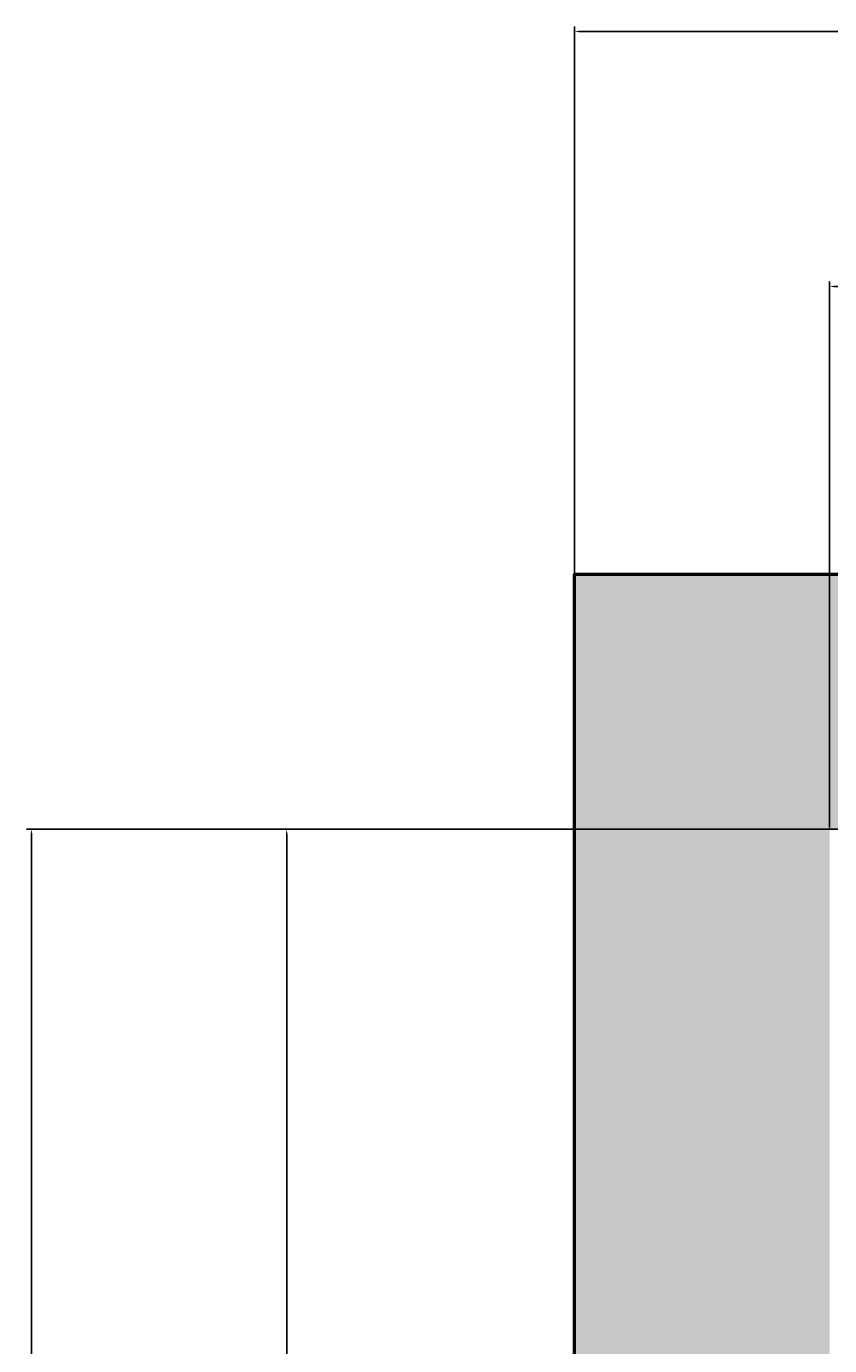
# Model space of a CAD drawing. Units: inches. Extents: x 2307 to 2544, y 2171 to 2540.
# Tile 23 of 52: x 2307 to 2336, y 2493 to 2540. Entities that reach past the tile are written whole.
import ezdxf

# ---------------------------------------------------------------- set-up
doc = ezdxf.new("R2010")
doc.units = ezdxf.units.IN
doc.layers.add('A-ANNO-DIMS', color=2, linetype='Continuous', lineweight=18)
doc.layers.add('A-WALL', color=7, linetype='Continuous', lineweight=50)
doc.layers.add('A-WALL-PATT', color=18, linetype='Continuous', lineweight=13, true_color=0x000000)
doc.styles.get("Standard").update_dxf_attribs({"font": 'arial.ttf'})
doc.dimstyles.get("Standard").update_dxf_attribs({"dimtxt": 0.18, "dimasz": 0.18, "dimexe": 0.18, "dimexo": 0.0625, "dimgap": 0.09, "dimtad": 0, "dimtih": 1, "dimtoh": 1, "dimdec": 4, "dimzin": 0, "dimdsep": 46, "dimtxsty": 'Standard', "dimcen": 0.09, "dimadec": 0, "dimazin": 0, "dimtfac": 1, "dimtdec": 4, "dimtofl": 0, "dimtmove": 0, "dimatfit": 3, "dimfxl": 1, "dimtolj": 1, "dimtzin": 0, "dimarcsym": 0})

# ---------------------------------------------------------------- blocks, each defined once
blk = doc.blocks.new('*D42')
at = {"layer": 'A-ANNO-DIMS', "color": 0, "lineweight": -2, "transparency": 16777216}
for p, q in [((2326.696, 2520.572), (2326.696, 2539.84)), ((2326.876, 2539.66), (2346.669, 2539.66)), ((2367.223, 2539.66), (2347.429, 2539.66)), ((2367.403, 2520.572), (2367.403, 2539.84))]:
    blk.add_line(p, q, dxfattribs=at)
at = {"layer": 'A-ANNO-DIMS', "color": 0, "transparency": 16777216}
for points in [[(2326.876, 2539.69), (2326.876, 2539.63), (2326.696, 2539.66)], [(2367.223, 2539.69), (2367.223, 2539.63), (2367.403, 2539.66)]]:
    blk.add_solid(points, dxfattribs=at)
at = {"layer": 'Defpoints', "color": 0, "transparency": 16777216}
for p in [(2367.403, 2539.66), (2326.696, 2520.51), (2367.403, 2520.51)]:
    blk.add_point(p, dxfattribs=at)
at = {"layer": 'A-ANNO-DIMS', "color": 0, "transparency": 16777216, "insert": (2347.049, 2539.66), "char_height": 0.18, "attachment_point": 5}
blk.add_mtext('\\A1;40.71', dxfattribs=at)
blk = doc.blocks.new('*D45')
at = {"layer": 'A-ANNO-DIMS', "color": 0, "lineweight": -2, "transparency": 16777216}
for p, q in [((2335.696, 2511.572), (2335.696, 2530.84)), ((2451.696, 2511.572), (2451.696, 2530.84)), ((2335.876, 2530.66), (2393.416, 2530.66)), ((2451.516, 2530.66), (2393.976, 2530.66))]:
    blk.add_line(p, q, dxfattribs=at)
at = {"layer": 'A-ANNO-DIMS', "color": 0, "transparency": 16777216}
for points in [[(2335.876, 2530.69), (2335.876, 2530.63), (2335.696, 2530.66)], [(2451.516, 2530.69), (2451.516, 2530.63), (2451.696, 2530.66)]]:
    blk.add_solid(points, dxfattribs=at)
at = {"layer": 'Defpoints', "color": 0, "transparency": 16777216}
for p in [(2451.696, 2530.66), (2335.696, 2511.51), (2451.696, 2511.51)]:
    blk.add_point(p, dxfattribs=at)
at = {"layer": 'A-ANNO-DIMS', "color": 0, "transparency": 16777216, "insert": (2393.696, 2530.66), "char_height": 0.18, "attachment_point": 5}
blk.add_mtext('\\A1;116', dxfattribs=at)
blk = doc.blocks.new('*D47')
at = {"layer": 'A-ANNO-DIMS', "color": 0, "lineweight": -2, "transparency": 16777216}
for p, q in [((2335.633, 2511.51), (2316.366, 2511.51)), ((2316.546, 2511.33), (2316.546, 2451.691)), ((2316.546, 2391.69), (2316.546, 2451.328)), ((2335.633, 2391.51), (2316.366, 2391.51))]:
    blk.add_line(p, q, dxfattribs=at)
at = {"layer": 'A-ANNO-DIMS', "color": 0, "transparency": 16777216}
for points in [[(2316.516, 2511.33), (2316.576, 2511.33), (2316.546, 2511.51)], [(2316.516, 2391.69), (2316.576, 2391.69), (2316.546, 2391.51)]]:
    blk.add_solid(points, dxfattribs=at)
at = {"layer": 'Defpoints', "color": 0, "transparency": 16777216}
for p in [(2316.546, 2511.51), (2335.696, 2511.51), (2335.696, 2391.51)]:
    blk.add_point(p, dxfattribs=at)
at = {"layer": 'A-ANNO-DIMS', "color": 0, "transparency": 16777216, "insert": (2316.546, 2451.51), "char_height": 0.18, "attachment_point": 5}
blk.add_mtext('\\A1;120', dxfattribs=at)
blk = doc.blocks.new('*D48')
at = {"layer": 'A-ANNO-DIMS', "color": 0, "lineweight": -2, "transparency": 16777216}
for p, q in [((2455.633, 2511.51), (2307.366, 2511.51)), ((2307.546, 2511.33), (2307.546, 2475.69)), ((2307.546, 2439.69), (2307.546, 2475.329)), ((2455.633, 2439.51), (2307.366, 2439.51))]:
    blk.add_line(p, q, dxfattribs=at)
at = {"layer": 'A-ANNO-DIMS', "color": 0, "transparency": 16777216}
for points in [[(2307.516, 2511.33), (2307.576, 2511.33), (2307.546, 2511.51)], [(2307.516, 2439.69), (2307.576, 2439.69), (2307.546, 2439.51)]]:
    blk.add_solid(points, dxfattribs=at)
at = {"layer": 'Defpoints', "color": 0, "transparency": 16777216}
for p in [(2307.546, 2511.51), (2455.696, 2511.51), (2455.696, 2439.51)]:
    blk.add_point(p, dxfattribs=at)
at = {"layer": 'A-ANNO-DIMS', "color": 0, "transparency": 16777216, "insert": (2307.546, 2475.51), "char_height": 0.18, "attachment_point": 5}
blk.add_mtext('\\A1;72', dxfattribs=at)

msp = doc.modelspace()

# ---------------------------------------------------------------- hatches: boundary and pattern name
at = {"layer": 'A-WALL-PATT'}
h = msp.add_hatch(color=256, dxfattribs=at)
h.dxf.hatch_style = 1
h.paths.add_polyline_path([(2367.4028, 2520.5096), (2326.6958, 2520.5096), (2326.6958, 2355.3983), (2335.6958, 2355.3983), (2335.6958, 2387.5096), (2415.6958, 2387.5096), (2415.6958, 2391.5096), (2335.6958, 2391.5096), (2335.6958, 2409.5096), (2335.6958, 2511.5096), (2367.4028, 2511.5096)])

# ---------------------------------------------------------------- linework, layer by layer
at = {"layer": 'A-WALL'}
msp.add_lwpolyline([(2433.7832, 2190.5096), (2326.6958, 2190.5096), (2326.6958, 2520.5096), (2524.6958, 2520.5096), (2524.6958, 2190.5096), (2469.785, 2190.5096)], dxfattribs=at)

# ---------------------------------------------------------------- dimensions: what is measured, and where the dimension line sits
at = {"layer": 'A-ANNO-DIMS'}
for base, p1, p2, override, picture, middle in [((2367.4028, 2539.6596), (2326.6958, 2520.5096), (2367.4028, 2520.5096), {"dimdec": 2, "dimlfac": 1, "dimrnd": 0, "dimzin": 0, "dimdsep": 46, "dimlunit": 2}, '*D42', (2347.0493, 2539.6596)), ((2451.6958, 2530.6596), (2335.6958, 2511.5096), (2451.6958, 2511.5096), {"dimdec": 0, "dimlfac": 1, "dimrnd": 0, "dimzin": 0, "dimdsep": 46, "dimlunit": 2}, '*D45', (2393.6958, 2530.6596))]:
    dim = msp.add_linear_dim(base=base, p1=p1, p2=p2, dimstyle='Standard', override=override, dxfattribs=at)
    dim.commit()
    dim.dimension.update_dxf_attribs({"geometry": picture, "text_midpoint": middle})
for base, p1, p2, picture, middle in [((2307.5458, 2511.5096), (2455.6958, 2439.5096), (2455.6958, 2511.5096), '*D48', (2307.5458, 2475.5096)), ((2316.5458, 2511.5096), (2335.6958, 2391.5096), (2335.6958, 2511.5096), '*D47', (2316.5458, 2451.5096))]:
    dim = msp.add_linear_dim(base=base, p1=p1, p2=p2, angle=90, dimstyle='Standard', override={"dimdec": 0, "dimlfac": 1, "dimrnd": 0, "dimzin": 0, "dimdsep": 46, "dimlunit": 2}, dxfattribs=at)
    dim.commit()
    dim.dimension.update_dxf_attribs({"geometry": picture, "text_midpoint": middle})

doc.saveas('drawing.dxf')
